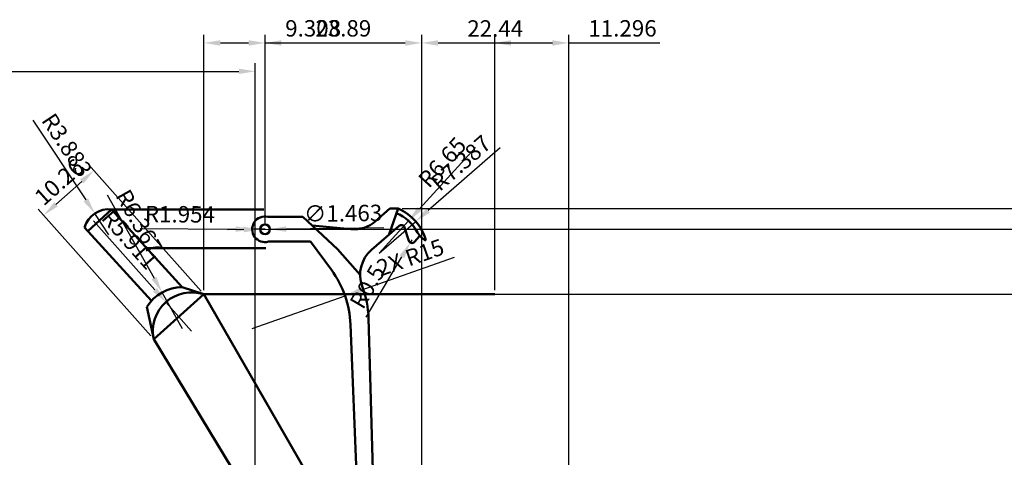
# Model space of a CAD drawing. Units: millimetres. Extents: x 1068 to 1546, y 1743 to 2032.
# Tile 8 of 9: x 1318 to 1469, y 1965 to 2032. Entities that reach past the tile are written whole.
import ezdxf

# ---------------------------------------------------------------- set-up
doc = ezdxf.new("R2010")
doc.units = ezdxf.units.MM
doc.layers.add('M-DIMS', color=2, linetype='Continuous', lineweight=25)
doc.layers.add('M-OUTL', color=7, linetype='Continuous', lineweight=50)
doc.styles.get("Standard").update_dxf_attribs({"font": 'arial.ttf'})
doc.dimstyles.new('ISO-25', dxfattribs={"dimtxt": 2.5, "dimasz": 2.5, "dimexe": 1.25, "dimexo": 0.625, "dimtad": 1, "dimtxsty": 'Standard', "dimcen": 2.5, "dimadec": 0, "dimazin": 0, "dimtfac": 1, "dimtmove": 0, "dimatfit": 3, "dimfxl": 1, "dimarcsym": 0})

# ---------------------------------------------------------------- blocks, each defined once
blk = doc.blocks.new('*D22')
at = {"layer": 'Defpoints', "color": 0, "transparency": 16777216}
for p in [(1354.41, 2023.87), (1212.56, 1957.56), (1354.41, 1957.56)]:
    blk.add_point(p, dxfattribs=at)
at = {"layer": 'M-DIMS', "color": 0, "lineweight": -2, "transparency": 16777216}
for p, q in [((1212.56, 1958.19), (1212.56, 2025.12)), ((1354.41, 1958.19), (1354.41, 2025.12)), ((1215.06, 2023.87), (1351.91, 2023.87))]:
    blk.add_line(p, q, dxfattribs=at)
at = {"layer": 'M-DIMS', "color": 0, "transparency": 16777216}
for points in [[(1215.06, 2024.29), (1215.06, 2023.46), (1212.56, 2023.87)], [(1351.91, 2024.29), (1351.91, 2023.46), (1354.41, 2023.87)]]:
    blk.add_solid(points, dxfattribs=at)
at = {"layer": 'M-DIMS', "color": 0, "transparency": 16777216, "insert": (1283.48, 2026), "char_height": 2.5, "attachment_point": 5}
blk.add_mtext('141,85', dxfattribs=at)
blk = doc.blocks.new('*D25')
at = {"layer": 'Defpoints', "color": 0, "transparency": 16777216}
for p in [(1376.21, 2002.95), (1507.48, 2002.95), (1402.23, 1769.76)]:
    blk.add_point(p, dxfattribs=at)
at = {"layer": 'M-DIMS', "color": 0, "lineweight": -2, "transparency": 16777216}
for p, q in [((1376.84, 2002.95), (1508.73, 2002.95)), ((1507.48, 1772.26), (1507.48, 2000.45)), ((1402.85, 1769.76), (1508.73, 1769.76))]:
    blk.add_line(p, q, dxfattribs=at)
at = {"layer": 'M-DIMS', "color": 0, "transparency": 16777216}
for points in [[(1507.06, 2000.45), (1507.89, 2000.45), (1507.48, 2002.95)], [(1507.06, 1772.26), (1507.89, 1772.26), (1507.48, 1769.76)]]:
    blk.add_solid(points, dxfattribs=at)
at = {"layer": 'M-DIMS', "color": 0, "transparency": 16777216, "insert": (1505.58, 1886.35), "char_height": 2.5, "attachment_point": 5, "rotation": 90}
blk.add_mtext('233.2', dxfattribs=at)
blk = doc.blocks.new('*D36')
at = {"layer": 'Defpoints', "color": 0, "transparency": 16777216}
for p in [(1346.59, 1989.88), (1507.48, 1989.88), (1354.41, 1957.56)]:
    blk.add_point(p, dxfattribs=at)
at = {"layer": 'M-DIMS', "color": 0, "lineweight": -2, "transparency": 16777216}
for p, q in [((1347.22, 1989.88), (1508.73, 1989.88)), ((1507.48, 1960.06), (1507.48, 1987.38)), ((1355.03, 1957.56), (1508.73, 1957.56))]:
    blk.add_line(p, q, dxfattribs=at)
at = {"layer": 'M-DIMS', "color": 0, "transparency": 16777216}
for points in [[(1507.06, 1987.38), (1507.89, 1987.38), (1507.48, 1989.88)], [(1507.06, 1960.06), (1507.89, 1960.06), (1507.48, 1957.56)]]:
    blk.add_solid(points, dxfattribs=at)
at = {"layer": 'M-DIMS', "color": 0, "transparency": 16777216, "insert": (1505.58, 1973.72), "char_height": 2.5, "attachment_point": 5, "rotation": 90}
blk.add_mtext('32.32', dxfattribs=at)
blk = doc.blocks.new('*D37')
at = {"layer": 'Defpoints', "color": 0, "transparency": 16777216}
for p in [(1355.9, 1999.79), (1507.48, 1999.79), (1346.59, 1989.88)]:
    blk.add_point(p, dxfattribs=at)
at = {"layer": 'M-DIMS', "color": 0, "lineweight": -2, "transparency": 16777216}
for p, q in [((1356.52, 1999.79), (1508.73, 1999.79)), ((1507.48, 1992.38), (1507.48, 1997.29)), ((1347.22, 1989.88), (1508.73, 1989.88))]:
    blk.add_line(p, q, dxfattribs=at)
at = {"layer": 'M-DIMS', "color": 0, "transparency": 16777216}
for points in [[(1507.06, 1997.29), (1507.89, 1997.29), (1507.48, 1999.79)], [(1507.06, 1992.38), (1507.89, 1992.38), (1507.48, 1989.88)]]:
    blk.add_solid(points, dxfattribs=at)
at = {"layer": 'M-DIMS', "color": 0, "transparency": 16777216, "insert": (1505.58, 1994.84), "char_height": 2.5, "attachment_point": 5, "rotation": 90}
blk.add_mtext('9.908', dxfattribs=at)
blk = doc.blocks.new('*D38')
at = {"layer": 'Defpoints', "color": 0, "transparency": 16777216}
for p in [(1355.9, 2028.2), (1355.9, 1999.79), (1346.59, 1989.88)]:
    blk.add_point(p, dxfattribs=at)
at = {"layer": 'M-DIMS', "color": 0, "lineweight": -2, "transparency": 16777216}
for p, q in [((1346.59, 1990.51), (1346.59, 2029.45)), ((1355.9, 2000.41), (1355.9, 2029.45)), ((1349.09, 2028.2), (1353.4, 2028.2)), ((1355.9, 2028.2), (1368.09, 2028.2))]:
    blk.add_line(p, q, dxfattribs=at)
at = {"layer": 'M-DIMS', "color": 0, "transparency": 16777216}
for points in [[(1349.09, 2028.61), (1349.09, 2027.78), (1346.59, 2028.2)], [(1353.4, 2028.61), (1353.4, 2027.78), (1355.9, 2028.2)]]:
    blk.add_solid(points, dxfattribs=at)
at = {"layer": 'M-DIMS', "color": 0, "transparency": 16777216, "insert": (1363.24, 2030.1), "char_height": 2.5, "attachment_point": 5}
blk.add_mtext('9.308', dxfattribs=at)
blk = doc.blocks.new('*D39')
at = {"layer": 'Defpoints', "color": 0, "transparency": 16777216}
for p in [(1379.79, 2028.2), (1355.9, 1999.79), (1379.79, 1936.04)]:
    blk.add_point(p, dxfattribs=at)
at = {"layer": 'M-DIMS', "color": 0, "lineweight": -2, "transparency": 16777216}
for p, q in [((1355.9, 2000.41), (1355.9, 2029.45)), ((1379.79, 1936.66), (1379.79, 2029.45)), ((1358.4, 2028.2), (1377.29, 2028.2))]:
    blk.add_line(p, q, dxfattribs=at)
at = {"layer": 'M-DIMS', "color": 0, "transparency": 16777216}
for points in [[(1358.4, 2028.61), (1358.4, 2027.78), (1355.9, 2028.2)], [(1377.29, 2028.61), (1377.29, 2027.78), (1379.79, 2028.2)]]:
    blk.add_solid(points, dxfattribs=at)
at = {"layer": 'M-DIMS', "color": 0, "transparency": 16777216, "insert": (1367.84, 2030.1), "char_height": 2.5, "attachment_point": 5}
blk.add_mtext('23.89', dxfattribs=at)
blk = doc.blocks.new('*D40')
at = {"layer": 'Defpoints', "color": 0, "transparency": 16777216}
for p in [(1402.23, 2028.2), (1379.79, 1936.04), (1402.23, 1849.76)]:
    blk.add_point(p, dxfattribs=at)
at = {"layer": 'M-DIMS', "color": 0, "lineweight": -2, "transparency": 16777216}
for p, q in [((1379.79, 1936.66), (1379.79, 2029.45)), ((1402.23, 1850.39), (1402.23, 2029.45)), ((1382.29, 2028.2), (1399.73, 2028.2))]:
    blk.add_line(p, q, dxfattribs=at)
at = {"layer": 'M-DIMS', "color": 0, "transparency": 16777216}
for points in [[(1382.29, 2028.61), (1382.29, 2027.78), (1379.79, 2028.2)], [(1399.73, 2028.61), (1399.73, 2027.78), (1402.23, 2028.2)]]:
    blk.add_solid(points, dxfattribs=at)
at = {"layer": 'M-DIMS', "color": 0, "transparency": 16777216, "insert": (1391.01, 2030.08), "char_height": 2.5, "attachment_point": 5}
blk.add_mtext('22.44', dxfattribs=at)
blk = doc.blocks.new('*D42')
at = {"layer": 'Defpoints', "color": 0, "transparency": 16777216}
for p in [(1329.81, 2008.75), (1346.59, 1989.88), (1338.92, 1983.06)]:
    blk.add_point(p, dxfattribs=at)
at = {"layer": 'M-DIMS', "color": 0, "lineweight": -2, "transparency": 16777216}
for p, q in [((1346.18, 1990.35), (1328.98, 2009.68)), ((1324.01, 2003.59), (1327.94, 2007.09)), ((1338.51, 1983.53), (1321.31, 2002.87))]:
    blk.add_line(p, q, dxfattribs=at)
at = {"layer": 'M-DIMS', "color": 0, "transparency": 16777216}
for points in [[(1327.67, 2007.4), (1328.22, 2006.78), (1329.81, 2008.75)], [(1323.74, 2003.91), (1324.29, 2003.28), (1322.14, 2001.93)]]:
    blk.add_solid(points, dxfattribs=at)
at = {"layer": 'M-DIMS', "color": 0, "transparency": 16777216, "insert": (1324.71, 2006.76), "char_height": 2.5, "attachment_point": 5, "rotation": 41.6473}
blk.add_mtext('10.26', dxfattribs=at)
blk = doc.blocks.new('*D51')
at = {"layer": 'Defpoints', "color": 0, "transparency": 16777216}
for p in [(1402.23, 2028.2), (1390.93, 1989.88), (1402.23, 1849.76)]:
    blk.add_point(p, dxfattribs=at)
at = {"layer": 'M-DIMS', "color": 0, "lineweight": -2, "transparency": 16777216}
for p, q in [((1390.93, 1990.51), (1390.93, 2029.45)), ((1402.23, 1850.39), (1402.23, 2029.45)), ((1393.43, 2028.2), (1399.73, 2028.2)), ((1402.23, 2028.2), (1416.12, 2028.2))]:
    blk.add_line(p, q, dxfattribs=at)
at = {"layer": 'M-DIMS', "color": 0, "transparency": 16777216}
for points in [[(1393.43, 2028.61), (1393.43, 2027.78), (1390.93, 2028.2)], [(1399.73, 2028.61), (1399.73, 2027.78), (1402.23, 2028.2)]]:
    blk.add_solid(points, dxfattribs=at)
at = {"layer": 'M-DIMS', "color": 0, "transparency": 16777216, "insert": (1410.42, 2030.1), "char_height": 2.5, "attachment_point": 5}
blk.add_mtext('11.296', dxfattribs=at)
blk = doc.blocks.new('*D68')
at = {"layer": 'Defpoints', "color": 0, "transparency": 16777216}
for p in [(1368.11, 1989.65), (1353.95, 1984.69)]:
    blk.add_point(p, dxfattribs=at)
at = {"layer": 'M-DIMS', "color": 0, "lineweight": -2, "transparency": 16777216}
for p, q in [((1384.77, 1995.5), (1370.47, 1990.48)), ((1353.95, 1984.69), (1368.11, 1989.65))]:
    blk.add_line(p, q, dxfattribs=at)
at = {"layer": 'M-DIMS', "color": 0, "transparency": 16777216}
blk.add_solid([(1370.33, 1990.87), (1370.6, 1990.09), (1368.11, 1989.65)], dxfattribs=at)
at = {"layer": 'M-DIMS', "color": 0, "transparency": 16777216, "insert": (1378.17, 1995.2), "char_height": 2.5, "attachment_point": 5, "rotation": 19.3418}
blk.add_mtext('2X R15', dxfattribs=at)
blk = doc.blocks.new('*D72')
at = {"layer": 'Defpoints', "color": 0, "transparency": 16777216}
for p in [(1378.89, 2001), (1373.31, 1996.15)]:
    blk.add_point(p, dxfattribs=at)
at = {"layer": 'M-DIMS', "color": 0, "lineweight": -2, "transparency": 16777216}
for p, q in [((1391.78, 2012.2), (1380.78, 2002.64)), ((1373.31, 1996.15), (1378.89, 2001))]:
    blk.add_line(p, q, dxfattribs=at)
at = {"layer": 'M-DIMS', "color": 0, "transparency": 16777216}
blk.add_solid([(1380.5, 2002.95), (1381.05, 2002.32), (1378.89, 2001)], dxfattribs=at)
at = {"layer": 'M-DIMS', "color": 0, "transparency": 16777216, "insert": (1385.97, 2009.67), "char_height": 2.5, "attachment_point": 5, "rotation": 40.9907}
blk.add_mtext('R7.387', dxfattribs=at)
blk = doc.blocks.new('*D73')
at = {"layer": 'Defpoints', "color": 0, "transparency": 16777216}
for p in [(1377.79, 2001.07), (1373.31, 1996.15)]:
    blk.add_point(p, dxfattribs=at)
at = {"layer": 'M-DIMS', "color": 0, "lineweight": -2, "transparency": 16777216}
for p, q in [((1387.99, 2012.28), (1379.47, 2002.92)), ((1373.31, 1996.15), (1377.79, 2001.07))]:
    blk.add_line(p, q, dxfattribs=at)
at = {"layer": 'M-DIMS', "color": 0, "transparency": 16777216}
blk.add_solid([(1379.16, 2003.2), (1379.78, 2002.64), (1377.79, 2001.07)], dxfattribs=at)
at = {"layer": 'M-DIMS', "color": 0, "transparency": 16777216, "insert": (1383.17, 2009.8), "char_height": 2.5, "attachment_point": 5, "rotation": 47.691}
blk.add_mtext('R6.65', dxfattribs=at)
blk = doc.blocks.new('*D74')
at = {"layer": 'Defpoints', "color": 0, "transparency": 16777216}
for p in [(1340.2, 1990.17), (1343.32, 1984.62)]:
    blk.add_point(p, dxfattribs=at)
at = {"layer": 'M-DIMS', "color": 0, "lineweight": -2, "transparency": 16777216}
for p, q in [((1331.83, 2005.06), (1338.97, 1992.35)), ((1343.32, 1984.62), (1340.2, 1990.17))]:
    blk.add_line(p, q, dxfattribs=at)
at = {"layer": 'M-DIMS', "color": 0, "transparency": 16777216}
blk.add_solid([(1339.34, 1992.56), (1338.61, 1992.15), (1340.2, 1990.17)], dxfattribs=at)
at = {"layer": 'M-DIMS', "color": 0, "transparency": 16777216, "insert": (1336.45, 2000.73), "char_height": 2.5, "attachment_point": 5, "rotation": 299.3585}
blk.add_mtext('R6.367', dxfattribs=at)
blk = doc.blocks.new('*D75')
at = {"layer": 'Defpoints', "color": 0, "transparency": 16777216}
for p in [(1340.78, 1988.7), (1344.71, 1984.28)]:
    blk.add_point(p, dxfattribs=at)
at = {"layer": 'M-DIMS', "color": 0, "lineweight": -2, "transparency": 16777216}
for p, q in [((1329.75, 2001.1), (1339.12, 1990.56)), ((1344.71, 1984.28), (1340.78, 1988.7))]:
    blk.add_line(p, q, dxfattribs=at)
at = {"layer": 'M-DIMS', "color": 0, "transparency": 16777216}
blk.add_solid([(1339.43, 1990.84), (1338.81, 1990.29), (1340.78, 1988.7)], dxfattribs=at)
at = {"layer": 'M-DIMS', "color": 0, "transparency": 16777216, "insert": (1335.03, 1998.03), "char_height": 2.5, "attachment_point": 5, "rotation": 311.6497}
blk.add_mtext('R5.911', dxfattribs=at)
blk = doc.blocks.new('*D78')
at = {"layer": 'Defpoints', "color": 0, "transparency": 16777216}
for p in [(1329.95, 2002.2), (1332.09, 1998.97)]:
    blk.add_point(p, dxfattribs=at)
at = {"layer": 'M-DIMS', "color": 0, "lineweight": -2, "transparency": 16777216}
for p, q in [((1320.49, 2016.43), (1328.56, 2004.28)), ((1332.09, 1998.97), (1329.95, 2002.2))]:
    blk.add_line(p, q, dxfattribs=at)
at = {"layer": 'M-DIMS', "color": 0, "transparency": 16777216}
blk.add_solid([(1328.91, 2004.51), (1328.21, 2004.05), (1329.95, 2002.2)], dxfattribs=at)
at = {"layer": 'M-DIMS', "color": 0, "transparency": 16777216, "insert": (1325.42, 2012.45), "char_height": 2.5, "attachment_point": 5, "rotation": 303.6032}
blk.add_mtext('R3.883', dxfattribs=at)
blk = doc.blocks.new('*D81')
at = {"layer": 'Defpoints', "color": 0, "transparency": 16777216}
for p in [(1355.17, 1999.78), (1356.63, 1999.8)]:
    blk.add_point(p, dxfattribs=at)
at = {"layer": 'M-DIMS', "color": 0, "lineweight": -2, "transparency": 16777216}
for p, q in [((1352.67, 1999.75), (1350.17, 1999.72)), ((1355.17, 1999.78), (1356.63, 1999.8)), ((1374.03, 2000.01), (1359.13, 1999.83))]:
    blk.add_line(p, q, dxfattribs=at)
at = {"layer": 'M-DIMS', "color": 0, "transparency": 16777216}
for points in [[(1352.66, 2000.17), (1352.67, 1999.33), (1355.17, 1999.78)], [(1359.12, 2000.25), (1359.13, 1999.41), (1356.63, 1999.8)]]:
    blk.add_solid(points, dxfattribs=at)
at = {"layer": 'M-DIMS', "color": 0, "transparency": 16777216, "insert": (1367.81, 2001.91), "char_height": 2.5, "attachment_point": 5, "rotation": 0.6973}
blk.add_mtext('∅1.463', dxfattribs=at)
blk = doc.blocks.new('*D82')
at = {"layer": 'Defpoints', "color": 0, "transparency": 16777216}
for p in [(1353.94, 1999.8), (1355.9, 1999.79)]:
    blk.add_point(p, dxfattribs=at)
at = {"layer": 'M-DIMS', "color": 0, "lineweight": -2, "transparency": 16777216}
for p, q in [((1336.88, 1999.9), (1351.44, 1999.81)), ((1355.9, 1999.79), (1353.94, 1999.8))]:
    blk.add_line(p, q, dxfattribs=at)
at = {"layer": 'M-DIMS', "color": 0, "transparency": 16777216}
blk.add_solid([(1351.45, 2000.23), (1351.44, 1999.4), (1353.94, 1999.8)], dxfattribs=at)
at = {"layer": 'M-DIMS', "color": 0, "transparency": 16777216, "insert": (1342.92, 2001.76), "char_height": 2.5, "attachment_point": 5, "rotation": 359.6773}
blk.add_mtext('R1.954', dxfattribs=at)
blk = doc.blocks.new('*D83')
at = {"layer": 'Defpoints', "color": 0, "transparency": 16777216}
for p in [(1378.05, 1997.77), (1378.3, 1998.2)]:
    blk.add_point(p, dxfattribs=at)
at = {"layer": 'M-DIMS', "color": 0, "lineweight": -2, "transparency": 16777216}
for p, q in [((1378.3, 1998.2), (1378.05, 1997.77)), ((1371.35, 1986.38), (1376.78, 1995.61))]:
    blk.add_line(p, q, dxfattribs=at)
at = {"layer": 'M-DIMS', "color": 0, "transparency": 16777216}
blk.add_solid([(1376.42, 1995.82), (1377.14, 1995.4), (1378.05, 1997.77)], dxfattribs=at)
at = {"layer": 'M-DIMS', "color": 0, "transparency": 16777216, "insert": (1371.79, 1990.88), "char_height": 2.5, "attachment_point": 5, "rotation": 59.5382}
blk.add_mtext('R0.5', dxfattribs=at)

msp = doc.modelspace()

# ---------------------------------------------------------------- linework, layer by layer
at = {"layer": 'M-OUTL'}
for p, q in [((1332.5119, 2002.8283), (1328.8795, 1999.5213)), ((1343.2888, 1990.9904), (1332.5119, 2002.8283)), ((1332.5119, 2002.8283), (1355.7409, 2002.8283)), ((1356.3456, 2001.6919), (1361.6823, 2001.6919)), ((1361.6823, 2001.6919), (1366.9386, 1996.7759)), ((1372.7705, 2001.0308), (1374.9588, 2002.9476)), ((1376.2106, 2002.9476), (1374.8545, 1999.0391)), ((1374.9588, 2002.9476), (1376.2106, 2002.9476)), ((1363.096, 2000.3697), (1363.096, 2000.3697)), ((1363.096, 2000.3697), (1369.0079, 1999.8139)), ((1372.1344, 1996.6399), (1376.3675, 2000.3135)), ((1338.5769, 1988.8692), (1328.373, 2000.0776)), ((1377.1716, 2000.0879), (1377.8229, 1998.0469)), ((1378.6713, 1997.865), (1379.4444, 1998.7265)), ((1356.4291, 1997.9095), (1362.8362, 1997.9095)), ((1362.8362, 1997.9095), (1366.0223, 1993.5929)), ((1337.9004, 1996.9093), (1356.0361, 1996.9093)), ((1366.9386, 1996.7759), (1370.4115, 1992.8636)), ((1338.924, 1983.0643), (1346.5904, 1989.8822)), ((1346.5904, 1989.8822), (1343.2888, 1990.9904)), ((1346.5904, 1989.8822), (1375.8591, 1939.0334)), ((1346.5904, 1989.8822), (1390.9319, 1989.8822)), ((1338.924, 1983.0643), (1337.8973, 1987.9574)), ((1368.9422, 1985.2737), (1370.3848, 1948.5438)), ((1371.687, 1986.2339), (1372.8438, 1944.2719)), ((1366.9956, 1936.8189), (1338.924, 1983.0643))]:
    msp.add_line(p, q, dxfattribs=at)
msp.add_circle((1355.8981, 1999.7899), 0.7315, dxfattribs=at)
for centre, radius, start, end in [((1332.0939, 1998.968), 3.8828, 83.819396, 163.394448), ((1355.8981, 1999.7899), 1.954, 76.758793, 285.770164), ((1373.3128, 1996.1522), 6.6501, 28.482962, 66.90464), ((1373.3128, 1996.1522), 7.3874, 15.084941, 66.90464), ((1369.476, 2004.7919), 5, 264.628854, 311.216565), ((1376.6952, 1999.9358), 0.5, 17.698979, 130.951934), ((1381.7948, 2000.7543), 3, 208.482962, 243.274498), ((1378.2992, 1998.1989), 0.5, 197.698979, 318.097102), ((1375.4115, 1992.8636), 5, 130.951934, 200.619013), ((1353.9537, 1984.685), 15, 2.249265, 36.431362), ((1343.3215, 1984.6238), 6.3667, 90.294306, 148.425805), ((1344.7094, 1984.2781), 5.9114, 71.445223, 191.849368), ((1356.6927, 1985.8206), 15, 1.579088, 20.619013)]:
    msp.add_arc(centre, radius, start, end, dxfattribs=at)

# ---------------------------------------------------------------- dimensions: what is measured, and where the dimension line sits
at = {"layer": 'M-DIMS'}
for base, p1, p2, override, picture, middle in [((1355.8981, 2028.1976), (1346.5904, 1989.8822), (1355.8981, 1999.7899), {"dimdec": 3, "dimlfac": 1, "dimrnd": 0, "dimzin": 0, "dimdsep": 46, "dimlunit": 2}, '*D38', (1363.2437, 2030.0999)), ((1379.7864, 2028.1976), (1355.8981, 1999.7899), (1379.7864, 1936.0393), {"dimdec": 2, "dimlfac": 1, "dimrnd": 0, "dimzin": 0, "dimdsep": 46, "dimlunit": 2}, '*D39', (1367.8422, 2030.0999)), ((1402.2281, 2028.1976), (1379.7864, 1936.0393), (1402.2281, 1849.7623), {"dimdec": 2, "dimlfac": 1, "dimrnd": 0, "dimzin": 0, "dimdsep": 46, "dimlunit": 2}, '*D40', (1391.0073, 2030.0777)), ((1402.2281, 2028.1976), (1390.9319, 1989.8822), (1402.2281, 1849.7623), {"dimdec": 3, "dimlfac": 1, "dimrnd": 0, "dimzin": 0, "dimdsep": 46, "dimlunit": 2}, '*D51', (1410.4239, 2030.099)), ((1354.405, 2023.8738), (1212.5594, 1957.5607), (1354.405, 1957.5607), {"dimclrd": 0, "dimclre": 0, "dimclrt": 0}, '*D22', (1283.4822, 2026.0012))]:
    dim = msp.add_linear_dim(base=base, p1=p1, p2=p2, dimstyle='ISO-25', override=override, dxfattribs=at)
    dim.commit()
    dim.dimension.update_dxf_attribs({"geometry": picture, "text_midpoint": middle})
for center, mpoint, override, picture, middle in [((1332.0939, 1998.968), (1329.945, 2002.202), {"dimdec": 3, "dimlfac": 1, "dimrnd": 0, "dimzin": 0, "dimdsep": 46, "dimlunit": 2}, '*D78', (1325.4198, 2012.4494)), ((1373.3128, 1996.1522), (1378.8889, 2000.9979), {"dimdec": 3, "dimlfac": 1, "dimrnd": 0, "dimzin": 0, "dimdsep": 46, "dimlunit": 2}, '*D72', (1385.9739, 2009.6749)), ((1373.3128, 1996.1522), (1377.7891, 2001.0701), {"dimdec": 2, "dimlfac": 1, "dimrnd": 0, "dimzin": 0, "dimdsep": 46, "dimlunit": 2}, '*D73', (1383.1665, 2009.8027)), ((1343.3215, 1984.6238), (1340.2001, 1990.1728), {"dimdec": 3, "dimlfac": 1, "dimrnd": 0, "dimzin": 0, "dimdsep": 46, "dimlunit": 2}, '*D74', (1336.4458, 2000.727)), ((1355.8981, 1999.7899), (1353.9442, 1999.8009), {"dimdec": 3, "dimlfac": 1, "dimrnd": 0, "dimzin": 0, "dimdsep": 46, "dimlunit": 2}, '*D82', (1342.9208, 2001.7644)), ((1344.7094, 1984.2781), (1340.7808, 1988.6952), {"dimdec": 3, "dimlfac": 1, "dimrnd": 0, "dimzin": 0, "dimdsep": 46, "dimlunit": 2}, '*D75', (1335.0255, 1998.0274)), ((1378.2992, 1998.1989), (1378.0457, 1997.7679), {"dimdec": 1, "dimlfac": 1, "dimrnd": 0, "dimzin": 0, "dimdsep": 46, "dimlunit": 2}, '*D83', (1371.7901, 1990.8824))]:
    dim = msp.add_radius_dim(center=center, mpoint=mpoint, dimstyle='ISO-25', override=override, dxfattribs=at)
    dim.commit()
    dim.dimension.update_dxf_attribs({"geometry": picture, "text_midpoint": middle})
for base, p1, p2, angle, override, picture, middle in [((1329.8107, 2008.7503), (1338.924, 1983.0643), (1346.5904, 1989.8822), 41.647295, {"dimdec": 2, "dimlfac": 1, "dimrnd": 0, "dimzin": 0, "dimdsep": 46, "dimlunit": 2}, '*D42', (1324.7139, 2006.7621)), ((1507.4781, 2002.9476), (1402.2281, 1769.7623), (1376.2106, 2002.9476), 90, {"dimdec": 1, "dimlfac": 1, "dimrnd": 0, "dimzin": 0, "dimdsep": 46, "dimlunit": 2}, '*D25', (1505.5758, 1886.355)), ((1507.4781, 1999.7899), (1346.5904, 1989.8822), (1355.8981, 1999.7899), 90, {"dimdec": 3, "dimlfac": 1, "dimrnd": 0, "dimzin": 0, "dimdsep": 46, "dimlunit": 2}, '*D37', (1505.5767, 1994.836)), ((1507.4781, 1989.8822), (1354.405, 1957.5607), (1346.5904, 1989.8822), 90, {"dimdec": 2, "dimlfac": 1, "dimrnd": 0, "dimzin": 0, "dimdsep": 46, "dimlunit": 2}, '*D36', (1505.5758, 1973.7215))]:
    dim = msp.add_linear_dim(base=base, p1=p1, p2=p2, angle=angle, dimstyle='ISO-25', override=override, dxfattribs=at)
    dim.commit()
    dim.dimension.update_dxf_attribs({"geometry": picture, "text_midpoint": middle})
dim = msp.add_diameter_dim_2p(p1=(1355.1666, 1999.781), p2=(1356.6296, 1999.7988), dimstyle='ISO-25', override={"dimdec": 3, "dimlfac": 1, "dimrnd": 0, "dimzin": 0, "dimdsep": 46, "dimlunit": 2}, dxfattribs=at)
dim.commit()
dim.dimension.update_dxf_attribs({"geometry": '*D81', "text_midpoint": (1367.8318, 1999.9351), "dimtype": 163})
dim = msp.add_radius_dim(center=(1353.9537, 1984.685), mpoint=(1368.1071, 1989.653), text='2X <>', dimstyle='ISO-25', override={"dimdec": 0, "dimlfac": 1, "dimrnd": 0, "dimzin": 0, "dimdsep": 46, "dimlunit": 2}, dxfattribs=at)
dim.commit()
dim.dimension.update_dxf_attribs({"geometry": '*D68', "text_midpoint": (1378.1664, 1995.1992)})

doc.saveas('drawing.dxf')
